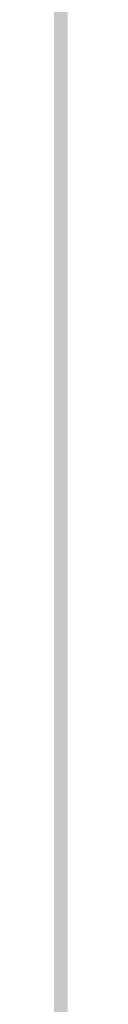
# Model space of a CAD drawing. Units: inches. Extents: x 2083 to 3317, y 1141 to 2115.
# Tile 182 of 256: x 3126.9594 to 3126.95969, y 1263.29018 to 1263.35483. Entities that reach past the tile are written whole.
import ezdxf

# ---------------------------------------------------------------- set-up
doc = ezdxf.new("R2010")
doc.units = ezdxf.units.IN
doc.layers.add('A-ANNO-DIMS', color=2, linetype='Continuous', lineweight=18)
doc.layers.add('A-WALL-PATT', color=251, linetype='Continuous', lineweight=13, true_color=0x636466)
doc.styles.get("Standard").update_dxf_attribs({"font": 'arial.ttf'})
doc.dimstyles.new('ISO-25', dxfattribs={"dimtxt": 12, "dimasz": 12, "dimexe": 1.25, "dimexo": 0.625, "dimtad": 1, "dimlunit": 3, "dimtxsty": 'Standard', "dimcen": 2.5, "dimadec": 0, "dimazin": 0, "dimtfac": 1, "dimtmove": 0, "dimatfit": 3, "dimfxl": 1, "dimarcsym": 0})

# ---------------------------------------------------------------- blocks, each defined once
blk = doc.blocks.new('*D26')
at = {"layer": 'A-ANNO-DIMS', "color": 0, "lineweight": -2, "transparency": 16777216}
for p, q in [((3088.985844, 1274.915092), (3088.985844, 1270.951963)), ((3111.240037, 1274.915092), (3111.240037, 1270.951963)), ((3076.985844, 1272.201963), (2840.262447, 1272.201963)), ((3111.240037, 1272.201963), (3088.985844, 1272.201963)), ((3123.240037, 1272.201963), (3135.240037, 1272.201963))]:
    blk.add_line(p, q, dxfattribs=at)
at = {"layer": 'A-ANNO-DIMS', "color": 0, "transparency": 16777216}
for points in [[(3076.985844, 1274.201963), (3076.985844, 1270.201963), (3088.985844, 1272.201963)], [(3123.240037, 1274.201963), (3123.240037, 1270.201963), (3111.240037, 1272.201963)]]:
    blk.add_solid(points, dxfattribs=at)
at = {"layer": 'Defpoints', "color": 0, "transparency": 16777216}
for p in [(3088.985844, 1275.540092), (3111.240037, 1275.540092), (3088.985844, 1272.201963)]:
    blk.add_point(p, dxfattribs=at)
at = {"layer": 'A-ANNO-DIMS', "color": 0, "transparency": 16777216, "insert": (2952.624146, 1279.031602), "char_height": 12, "attachment_point": 5}
blk.add_mtext('NIGHTSTAND 1\'-10 1/2" TYP.', dxfattribs=at)
blk = doc.blocks.new('*D27')
at = {"layer": 'A-ANNO-DIMS', "color": 0, "lineweight": -2, "transparency": 16777216}
for p, q in [((3114.578165, 1309.794285), (3114.578165, 1321.794285)), ((3111.865037, 1297.794285), (3115.828165, 1297.794285)), ((3114.578165, 1297.794285), (3114.578165, 1275.540092)), ((3111.865037, 1275.540092), (3115.828165, 1275.540092)), ((3114.578165, 1263.540092), (3114.578165, 1140.988591))]:
    blk.add_line(p, q, dxfattribs=at)
at = {"layer": 'A-ANNO-DIMS', "color": 0, "transparency": 16777216}
for points in [[(3112.578165, 1309.794285), (3116.578165, 1309.794285), (3114.578165, 1297.794285)], [(3112.578165, 1263.540092), (3116.578165, 1263.540092), (3114.578165, 1275.540092)]]:
    blk.add_solid(points, dxfattribs=at)
at = {"layer": 'Defpoints', "color": 0, "transparency": 16777216}
for p in [(3111.240037, 1297.794285), (3111.240037, 1275.540092), (3114.578165, 1275.540092)]:
    blk.add_point(p, dxfattribs=at)
at = {"layer": 'A-ANNO-DIMS', "color": 0, "transparency": 16777216, "insert": (3107.748527, 1196.264342), "char_height": 12, "attachment_point": 5, "rotation": 90}
blk.add_mtext('1\'-10 1/2" TYP.', dxfattribs=at)

msp = doc.modelspace()

# ---------------------------------------------------------------- hatches: boundary and pattern name
at = {"layer": 'A-WALL-PATT'}
h = msp.add_hatch(color=256, dxfattribs=at)
h.dxf.hatch_style = 1
h.paths.add_polyline_path([(3126.959783, 2020.76136), (2748.959783, 2020.76136), (2604.959783, 2020.76136), (2226.959783, 2020.76136), (2226.959783, 1702.76136), (2466.959783, 1702.76136), (2466.959783, 1582.76136), (2418.959783, 1582.76136), (2418.959783, 1477.76136), (2226.959783, 1477.76136), (2226.959783, 1263.26136), (2544.959783, 1263.26136), (2544.959783, 1411.76136), (2604.959783, 1411.76136), (2685.959783, 1411.76136), (2685.959783, 1420.76136), (2604.959783, 1420.76136), (2604.959783, 1573.76136), (2604.959783, 1702.76136), (2604.959783, 2011.76136), (2748.959783, 2011.76136), (2748.959783, 1702.76136), (2862.959783, 1702.76136), (2862.959783, 1621.76136), (2871.959783, 1621.76136), (2871.959783, 1702.76136), (2883.959783, 1702.76136), (2883.959783, 1706.939459, -0.026459), (2883.959783, 1711.76136), (2757.959783, 1711.76136), (2757.959783, 1807.76136), (2787.959783, 1807.76136), (2787.959783, 1812.26136), (2757.959783, 1812.26136), (2757.959783, 2011.76136), (2877.959783, 2011.76136), (2877.959783, 1812.26136), (2847.959783, 1812.26136), (2847.959783, 1807.76136), (2889.835742, 1807.76136), (2889.835742, 1812.26136), (2882.459783, 1812.26136), (2882.459783, 2011.76136), (3117.959783, 2011.76136), (3117.959783, 1812.26136), (2937.835742, 1812.26136), (2937.835742, 1807.76136), (2995.709783, 1807.76136), (2995.709783, 1796.117666), (3000.209783, 1796.117666), (3000.209783, 1807.76136), (3117.959783, 1807.76136), (3117.959783, 1711.76136), (3000.209783, 1711.76136), (3000.209783, 1760.117666), (2998.572705, 1760.117666, -0.020711), (2995.709783, 1760.117666), (2995.709783, 1711.76136), (2931.959783, 1711.76136), (2931.959783, 1702.76136), (3126.959783, 1702.76136)])
h.paths.add_polyline_path([(2471.459783, 2011.76136), (2471.459783, 1810.01136), (2462.716936, 1810.01136), (2462.716936, 1805.51136), (2505.959783, 1805.51136), (2505.959783, 1810.01136), (2475.959783, 1810.01136), (2475.959783, 2011.76136), (2595.959783, 2011.76136), (2595.959783, 1810.01136), (2565.959783, 1810.01136), (2565.959783, 1805.51136), (2595.959783, 1805.51136), (2595.959783, 1711.76136), (2235.959783, 1711.76136), (2235.959783, 1805.51136), (2353.709783, 1805.51136), (2353.709783, 1796.054162), (2358.209783, 1796.054162), (2358.209783, 1805.51136), (2414.716936, 1805.51136), (2414.716936, 1810.01136), (2235.959783, 1810.01136), (2235.959783, 2011.76136)], flags=16)
h.paths.add_polyline_path([(2270.204734, 1994.610008), (2270.204734, 1970.610008), (2246.204734, 1970.610008), (2246.204734, 1994.610008)], flags=0)
edge = h.paths.add_edge_path(flags=0)
edge.add_ellipse((2332.027391, 1899.798176), major_axis=(-3.042994, 3.042994), ratio=0.16825245, start_angle=-161.332166, end_angle=-156.307114, ccw=False)
edge.add_ellipse((2333.082037, 1898.74353), major_axis=(-1.054646, 1.054646), ratio=0.4535321, start_angle=-123.371019, end_angle=-94.159107)
edge = h.paths.add_edge_path(flags=0)
edge.add_ellipse((2332.027391, 1968.87629), major_axis=(3.042994, 3.042994), ratio=0.16825245, start_angle=18.667834, end_angle=23.692886)
edge.add_spline(control_points=[(2332.925596, 1970.691105), (2332.226768, 1970.3361), (2330.893709, 1969.658905), (2328.41308, 1970.932138), (2327.203934, 1967.748712), (2324.709596, 1969.955589), (2322.532822, 1967.012354), (2320.012846, 1971.295812), (2317.680308, 1968.157845), (2316.040526, 1967.102047), (2315.426904, 1966.809602)], knot_values=[0, 0, 0, 0, 2.267059, 4.324559, 6.685584, 8.878641, 11.121502, 14.300359, 17.755284, 19.732645, 19.732645, 19.732645, 19.732645], degree=3, periodic=0)
edge.add_ellipse((2332.027391, 1968.87629), major_axis=(3.042994, 3.042994), ratio=0.16825245, start_angle=18.667834, end_angle=23.692886, ccw=False)
edge.add_ellipse((2333.082037, 1969.930936), major_axis=(1.054646, 1.054646), ratio=0.4535321, start_angle=56.628981, end_angle=85.840893, ccw=False)
edge = h.paths.add_edge_path(flags=0)
edge.add_spline(control_points=[(2296.428287, 1967.987908), (2293.627804, 1965.336314), (2287.703624, 1959.727094), (2299.74386, 1949.995699), (2294.532591, 1935.668528), (2290.573228, 1920.603512), (2293.394124, 1909.973691), (2296.185407, 1904.966543)], knot_values=[0.099185, 0.099185, 0.099185, 0.099185, 0.345301, 0.619822, 0.982653, 1.386093, 1.810555, 1.810555, 1.810555, 1.810555], degree=3, periodic=0)
edge.add_spline(control_points=[(2296.185407, 1904.966543), (2297.383582, 1902.6193), (2298.000969, 1901.949312), (2298.55297, 1901.468155)], knot_values=[0.006246, 0.006246, 0.006246, 0.006246, 0.055476, 0.055476, 0.055476, 0.055476], degree=3, periodic=0)
edge.add_spline(control_points=[(2298.55297, 1901.468155), (2297.258612, 1900.923224), (2295.225294, 1900.232126), (2293.060229, 1900.614205), (2292.101423, 1900.788415), (2292.089578, 1900.790568)], knot_values=[0.312835, 0.312835, 0.312835, 0.312835, 0.40178, 0.474987, 0.475903, 0.475903, 0.475903, 0.475903], degree=3, periodic=0)
edge.add_arc((2292.793646, 1904.664109), 3.937008, 215.420897, 259.698179, ccw=False)
edge.add_spline(control_points=[(2289.585314, 1902.382304), (2289.476652, 1902.535087), (2289.36848, 1902.688035), (2289.260865, 1902.84117)], knot_values=[0.102872, 0.102872, 0.102872, 0.102872, 0.116896, 0.116896, 0.116896, 0.116896], degree=3, periodic=0)
edge.add_spline(control_points=[(2289.260865, 1902.84117), (2288.686604, 1902.550192), (2287.640048, 1902.019902), (2285.881337, 1901.873954), (2283.852972, 1901.504352), (2281.719987, 1899.710538), (2278.466991, 1899.492942), (2276.157136, 1901.883202), (2272.258953, 1899.804071), (2267.777605, 1901.843183), (2262.243882, 1900.184033), (2257.414927, 1901.782061), (2254.318374, 1900.72612), (2253.178285, 1900.337343)], knot_values=[0, 0, 0, 0, 1.907977, 3.477176, 5.261074, 7.972851, 11.680248, 13.717921, 16.939592, 22.789562, 27.502503, 33.595215, 37.145618, 37.145618, 37.145618, 37.145618], degree=3, periodic=0)
edge.add_line((2253.178285, 1900.337343), (2250.24424, 1902.84117))
edge.add_line((2250.24424, 1902.84117), (2250.24424, 1965.833296))
edge.add_line((2250.24424, 1965.833296), (2253.178285, 1968.337123))
edge.add_spline(control_points=[(2253.178285, 1968.337123), (2254.318374, 1967.948346), (2257.414927, 1966.892405), (2262.243882, 1968.490433), (2267.777605, 1966.831283), (2271.52673, 1968.537217), (2273.875914, 1967.828289), (2274.206701, 1967.727642)], knot_values=[0, 0, 0, 0, 0.09018, 0.244935, 0.364644, 0.513233, 0.537855, 0.537855, 0.537855, 0.537855], degree=3, periodic=0)
edge.add_arc((2274.352887, 1963.793349), 3.937008, 72.051134, 92.127949, ccw=False)
edge.add_arc((2281.296933, 1985.230003), 18.596298, 252.0511336, 288.5657217)
edge.add_arc((2292.316717, 1956.02888), 12.646081, 71.0267879, 113.7782184, ccw=False)
edge = h.paths.add_edge_path(flags=0)
edge.add_spline(control_points=[(2274.899415, 1951.856195), (2275.066156, 1951.616592), (2275.232687, 1951.376588), (2275.397987, 1951.135855)], knot_values=[1.409916, 1.409916, 1.409916, 1.409916, 1.43159, 1.43159, 1.43159, 1.43159], degree=3, periodic=0)
edge.add_spline(control_points=[(2275.397987, 1951.135855), (2275.792106, 1950.561885), (2276.179231, 1949.983774), (2276.545546, 1949.397103)], knot_values=[1.358238, 1.358238, 1.358238, 1.358238, 1.409916, 1.409916, 1.409916, 1.409916], degree=3, periodic=0)
edge.add_line((2276.545546, 1949.397103), (2277.437289, 1947.862185))
edge.add_spline(control_points=[(2277.437289, 1947.862185), (2276.303834, 1945.673115), (2274.639698, 1942.426882), (2274.631615, 1938.0939), (2272.799124, 1930.85155), (2274.356426, 1943.897046), (2275.947681, 1947.923356), (2276.545546, 1949.397103)], knot_values=[0.005632, 0.005632, 0.005632, 0.005632, 0.186014, 0.266002, 0.357087, 0.59639, 0.739732, 0.739732, 0.739732, 0.739732], degree=3, periodic=0)
edge.add_spline(control_points=[(2276.545546, 1949.397103), (2276.179231, 1949.983774), (2275.792106, 1950.561885), (2275.397987, 1951.135855)], knot_values=[1.358238, 1.358238, 1.358238, 1.358238, 1.409916, 1.409916, 1.409916, 1.409916], degree=3, periodic=0)
edge.add_spline(control_points=[(2275.397987, 1951.135855), (2274.9425, 1950.080452), (2274.20776, 1948.025272), (2273.934602, 1944.851477), (2272.468534, 1937.627489), (2273.466216, 1945.696466), (2274.700615, 1951.059472), (2274.899415, 1951.856195)], knot_values=[0.104364, 0.104364, 0.104364, 0.104364, 0.189636, 0.269624, 0.36071, 0.600013, 0.644622, 0.644622, 0.644622, 0.644622], degree=3, periodic=0)
h.paths.add_polyline_path([(2269.167514, 1963.127573, -0.357527), (2268.170633, 1960.97637, -0.092561), (2268.170633, 1939.436325, -0.357527), (2269.167514, 1937.285122, -0.357527), (2267.01631, 1938.282002, -0.164785), (2254.685581, 1938.282002, -0.357527), (2252.534378, 1937.285122, -0.357527), (2253.531259, 1939.436325, -0.092561), (2253.531259, 1960.97637, -0.357527), (2252.534378, 1963.127573, -0.357527), (2254.685581, 1962.130692, -0.164785), (2267.01631, 1962.130692, -0.357527)], flags=0)
h.paths.add_polyline_path([(2248.874068, 1967.8018), (2248.874068, 1957.02771), (2249.457783, 1957.02771), (2249.457783, 1911.646756), (2248.874068, 1911.646756), (2248.874068, 1900.872666), (2246.511863, 1900.872666, 0.197327), (2244.149658, 1902.456873), (2244.149658, 1966.217592, 0.197327), (2246.511863, 1967.8018)], flags=0)
h.paths.add_polyline_path([(2269.167514, 1931.389344, -0.357527), (2268.170633, 1929.238141, -0.092561), (2268.170633, 1907.698096, -0.357527), (2269.167514, 1905.546893, -0.357527), (2267.01631, 1906.543774, -0.164785), (2254.685581, 1906.543774, -0.357527), (2252.534378, 1905.546893, -0.357527), (2253.531259, 1907.698096, -0.092561), (2253.531259, 1929.238141, -0.357527), (2252.534378, 1931.389344, -0.357527), (2254.685581, 1930.392463, -0.164785), (2267.01631, 1930.392463, -0.357527)], flags=0)
edge = h.paths.add_edge_path(flags=0)
edge.add_spline(control_points=[(2276.196858, 1906.723702), (2276.168144, 1909.028928), (2276.114049, 1913.371852), (2270.598417, 1924.924978), (2273.905175, 1919.012779), (2275.921711, 1916.262063), (2275.47457, 1912.402149), (2277.257874, 1910.380621), (2276.696044, 1908.225036), (2276.646218, 1906.813023), (2276.617825, 1906.008407)], knot_values=[0, 0, 0, 0, 8.61026, 16.221274, 18.843057, 23.804898, 27.440828, 29.356102, 31.203478, 33.650687, 33.650687, 33.650687, 33.650687], degree=3, periodic=0)
edge.add_spline(control_points=[(2276.617825, 1906.008407), (2276.623313, 1905.624144), (2276.497738, 1904.628661), (2275.441779, 1903.854725), (2274.937314, 1903.08045), (2274.85908, 1902.84117)], knot_values=[0.156488, 0.156488, 0.156488, 0.156488, 0.184398, 0.231376, 0.250598, 0.250598, 0.250598, 0.250598], degree=3, periodic=0)
edge.add_line((2274.85908, 1902.84117), (2276.50598, 1902.84117))
edge.add_spline(control_points=[(2276.50598, 1902.84117), (2276.788308, 1903.08494), (2277.665071, 1904.125196), (2278.249538, 1904.340738), (2277.653872, 1908.527387), (2278.15567, 1906.227808), (2278.100464, 1905.285948), (2278.846675, 1904.069005), (2277.856785, 1903.414948), (2277.874191, 1902.99105), (2277.903562, 1902.84117)], knot_values=[0.059574, 0.059574, 0.059574, 0.059574, 0.080753, 0.103741, 0.16972, 0.176036, 0.207137, 0.240474, 0.262341, 0.27366, 0.27366, 0.27366, 0.27366], degree=3, periodic=0)
edge.add_line((2277.903562, 1902.84117), (2280.029825, 1902.84117))
edge.add_spline(control_points=[(2280.029825, 1902.84117), (2279.888221, 1903.088398), (2279.499257, 1903.981551), (2280.152284, 1905.939349), (2278.103615, 1909.657757), (2279.762395, 1907.185285), (2280.3279, 1904.874861), (2280.485109, 1903.48959), (2281.463269, 1903.249432), (2281.758343, 1902.936497), (2281.834036, 1902.84117)], knot_values=[0.013856, 0.013856, 0.013856, 0.013856, 0.034874, 0.088867, 0.107879, 0.126738, 0.158714, 0.193757, 0.217487, 0.226722, 0.226722, 0.226722, 0.226722], degree=3, periodic=0)
edge.add_spline(control_points=[(2281.834036, 1902.84117), (2281.787535, 1902.826703), (2281.647022, 1902.782988), (2281.395527, 1902.85949), (2281.088077, 1902.985242), (2280.720683, 1903.060902), (2280.333451, 1903.025726), (2280.124767, 1902.898879), (2280.029825, 1902.84117)], knot_values=[0, 0, 0, 0, 0.14413, 0.435517, 0.749276, 1.153046, 1.548371, 1.878348, 1.878348, 1.878348, 1.878348], degree=3, periodic=0)
edge.add_line((2280.029825, 1902.84117), (2277.903562, 1902.84117))
edge.add_spline(control_points=[(2277.903562, 1902.84117), (2277.892855, 1902.795855), (2277.865396, 1902.679637), (2277.607479, 1902.687483), (2277.27405, 1902.8007), (2276.837921, 1902.619775), (2276.583807, 1902.789261), (2276.50598, 1902.84117)], knot_values=[0, 0, 0, 0, 0.127189, 0.326199, 0.628009, 1.24357, 1.515331, 1.515331, 1.515331, 1.515331], degree=3, periodic=0)
edge.add_line((2276.50598, 1902.84117), (2274.85908, 1902.84117))
edge.add_spline(control_points=[(2274.85908, 1902.84117), (2274.814437, 1902.898587), (2274.72513, 1903.013446), (2274.493477, 1903.118968), (2274.244285, 1902.960539), (2273.937121, 1903.184942), (2273.614039, 1902.983143), (2273.408316, 1902.883045), (2273.322254, 1902.84117)], knot_values=[0, 0, 0, 0, 0.21843, 0.436957, 0.687977, 0.990379, 1.398396, 1.69185, 1.69185, 1.69185, 1.69185], degree=3, periodic=0)
edge.add_spline(control_points=[(2273.322254, 1902.84117), (2273.61674, 1903.445692), (2274.273998, 1904.538253), (2276.027239, 1904.573702), (2276.206963, 1906.583637), (2276.196858, 1906.723702)], knot_values=[0.012227, 0.012227, 0.012227, 0.012227, 0.059472, 0.106218, 0.134458, 0.134458, 0.134458, 0.134458], degree=3, periodic=0)
h.paths.add_polyline_path([(2270.776054, 1897.789828), (2270.776054, 1873.789828), (2246.776054, 1873.789828), (2246.776054, 1897.789828)], flags=0)
h.paths.add_polyline_path([(2353.709783, 1760.005059), (2353.709783, 1760.054162), (2358.209783, 1760.054162, -0.033729)], flags=0)
h.paths.add_polyline_path([(2321.819119, 1737.529186), (2341.995327, 1737.529186, -0.414214), (2343.203273, 1736.321241), (2343.203273, 1721.020596, -0.414214), (2341.995327, 1719.812651), (2321.819119, 1719.812651, -0.414214), (2320.611173, 1721.020596), (2320.611173, 1736.321241, -0.414214)], flags=0)
h.paths.add_polyline_path([(2324.23501, 1736.321241), (2339.579436, 1736.321241, -0.414214), (2341.995327, 1733.905349), (2341.995327, 1725.44973, -0.414214), (2339.579436, 1723.033839), (2333.680588, 1723.033839), (2333.845317, 1722.045467, -0.870646), (2335.425399, 1721.825893, -0.767327), (2333.922694, 1721.423245), (2331.291024, 1721.423245, -0.767327), (2329.788319, 1721.825893, -0.870646), (2331.368401, 1722.045467), (2331.53313, 1723.033839), (2324.23501, 1723.033839, -0.414214), (2321.819119, 1725.44973), (2321.819119, 1733.905349, -0.414214)], flags=0)
h.paths.add_polyline_path([(2570.483789, 1928.615444), (2589.683789, 1928.615444), (2590.168829, 1928.615444), (2590.168829, 1904.993397), (2570.483789, 1904.993397)], flags=0)
h.paths.add_polyline_path([(2574.447324, 1927.263822, -1), (2572.828836, 1927.263822, -1)], flags=0)
h.paths.add_polyline_path([(2573.089867, 1926.940877), (2573.925032, 1927.776042), (2574.147743, 1927.553332), (2573.312577, 1926.718166)], flags=0)
h.paths.add_polyline_path([(2578.779065, 1919.729618, -1), (2571.591663, 1919.729618, -1)], flags=0)
h.paths.add_polyline_path([(2578.385364, 1919.729618, -1), (2571.985364, 1919.729618, -1)], flags=0)
h.paths.add_polyline_path([(2331.595764, 1729.476216, -1), (2333.617954, 1729.476216, -1)], flags=0)
h.paths.add_polyline_path([(2578.034228, 1927.263822, -1), (2576.41574, 1927.263822, -1)], flags=0)
h.paths.add_polyline_path([(2576.688851, 1927.531089), (2576.911562, 1927.753799), (2577.746728, 1926.918634), (2577.524017, 1926.695923)], flags=0)
h.paths.add_polyline_path([(2578.139065, 1909.859539, -1), (2572.231663, 1909.859539, -1)], flags=0)
h.paths.add_polyline_path([(2577.745364, 1909.859539, -1), (2572.625364, 1909.859539, -1)], flags=0)
h.paths.add_polyline_path([(2583.797718, 1927.263822, -1), (2582.179229, 1927.263822, -1)], flags=0)
h.paths.add_polyline_path([(2582.718649, 1927.753799), (2583.553814, 1926.918634), (2583.331103, 1926.695923), (2582.495938, 1927.531089)], flags=0)
h.paths.add_polyline_path([(2582.495938, 1927.531089), (2582.718649, 1927.753799), (2583.553814, 1926.918634), (2583.331103, 1926.695923)], flags=0)
h.paths.add_polyline_path([(2587.739065, 1920.529618, -1), (2581.831663, 1920.529618, -1)], flags=0)
h.paths.add_polyline_path([(2587.345364, 1920.529618, -1), (2582.225364, 1920.529618, -1)], flags=0)
h.paths.add_polyline_path([(2587.384622, 1927.263822, -1), (2585.766133, 1927.263822, -1)], flags=0)
h.paths.add_polyline_path([(2586.081993, 1926.980247), (2586.917158, 1927.815412), (2587.139869, 1927.592702), (2586.304703, 1926.757536)], flags=0)
h.paths.add_polyline_path([(2588.379065, 1910.659539, -1), (2581.191663, 1910.659539, -1)], flags=0)
h.paths.add_polyline_path([(2587.985364, 1910.659539, -1), (2581.585364, 1910.659539, -1)], flags=0)
h.paths.add_polyline_path([(2417.167729, 1729.477895), (2437.343937, 1729.477895, -0.414214), (2438.551883, 1728.26995), (2438.551883, 1712.969306, -0.414214), (2437.343937, 1711.76136), (2417.167729, 1711.76136, -0.414214), (2415.959783, 1712.969306), (2415.959783, 1728.26995, -0.414214)], flags=0)
h.paths.add_polyline_path([(2419.58362, 1728.26995), (2434.928046, 1728.26995, -0.414214), (2437.343937, 1725.854059), (2437.343937, 1717.39844, -0.414214), (2434.928046, 1714.982548), (2429.029199, 1714.982548), (2429.193927, 1713.994176, -0.870646), (2430.774009, 1713.774603, -0.767327), (2429.271304, 1713.371954), (2426.639634, 1713.371954, -0.767327), (2425.136929, 1713.774603, -0.870646), (2426.717011, 1713.994176), (2426.88174, 1714.982548), (2419.58362, 1714.982548, -0.414214), (2417.167729, 1717.39844), (2417.167729, 1725.854059, -0.414214)], flags=0)
h.paths.add_polyline_path([(2419.58362, 1728.26995), (2434.928046, 1728.26995, -0.414214), (2437.343937, 1725.854059), (2437.343937, 1717.39844, -0.414214), (2434.928046, 1714.982548), (2429.029199, 1714.982548), (2428.358118, 1719.009034), (2427.552821, 1719.009034), (2426.88174, 1714.982548), (2419.58362, 1714.982548, -0.414214), (2417.167729, 1717.39844), (2417.167729, 1725.854059, -0.414214)], flags=0)
h.paths.add_polyline_path([(2426.944374, 1721.424925, -1), (2428.966564, 1721.424925, -1)], flags=0)
h.paths.add_polyline_path([(2475.959783, 1702.76136), (2595.959783, 1702.76136), (2595.959783, 1582.76136), (2475.959783, 1582.76136)], flags=16)
h.paths.add_polyline_path([(2427.959783, 1573.76136), (2595.959783, 1573.76136), (2595.959783, 1468.76136), (2595.959783, 1420.76136), (2384.459783, 1420.76136), (2384.459783, 1468.76136), (2427.959783, 1468.76136)], flags=16)
h.paths.add_polyline_path([(2379.959783, 1468.76136), (2379.959783, 1420.76136), (2235.959783, 1420.76136), (2235.959783, 1468.76136)], flags=16)
h.paths.add_polyline_path([(2317.815996, 1466.695767), (2337.992205, 1466.695767, -0.414214), (2339.20015, 1465.487821), (2339.20015, 1450.187177, -0.414214), (2337.992205, 1448.979232), (2317.815996, 1448.979232, -0.414214), (2316.608051, 1450.187177), (2316.608051, 1465.487821, -0.414214)], flags=0)
h.paths.add_polyline_path([(2320.231887, 1465.487821), (2335.576313, 1465.487821, -0.414214), (2337.992205, 1463.07193), (2337.992205, 1454.616311, -0.414214), (2335.576313, 1452.20042), (2329.677466, 1452.20042), (2329.842195, 1451.212047, -0.870646), (2331.422276, 1450.992474, -0.767327), (2329.919571, 1450.589826), (2327.287902, 1450.589826, -0.767327), (2325.785197, 1450.992474, -0.870646), (2327.365278, 1451.212047), (2327.530007, 1452.20042), (2320.231887, 1452.20042, -0.414214), (2317.815996, 1454.616311), (2317.815996, 1463.07193, -0.414214)], flags=0)
h.paths.add_polyline_path([(2320.231887, 1465.487821), (2335.576313, 1465.487821, -0.414214), (2337.992205, 1463.07193), (2337.992205, 1454.616311, -0.414214), (2335.576313, 1452.20042), (2329.677466, 1452.20042), (2329.006385, 1456.226905), (2328.201088, 1456.226905), (2327.530007, 1452.20042), (2320.231887, 1452.20042, -0.414214), (2317.815996, 1454.616311), (2317.815996, 1463.07193, -0.414214)], flags=0)
h.paths.add_polyline_path([(2327.592641, 1458.642796, -1), (2329.614832, 1458.642796, -1)], flags=0)
h.paths.add_polyline_path([(2244.411744, 1433.340453), (2241.920945, 1433.340453, -0.414214), (2240.017856, 1435.243542), (2240.017856, 1440.952808, -0.414211), (2241.920925, 1442.855897), (2244.411744, 1442.855897, -1.976472)], flags=0)
h.paths.add_polyline_path([(2245.356888, 1434.397536, -0.414214), (2245.356888, 1441.798814, -2.144098)], flags=0)
h.paths.add_polyline_path([(2535.959783, 1416.26136), (2535.959783, 1272.26136), (2235.959783, 1272.26136), (2235.959783, 1416.26136)], flags=16)
h.paths.add_polyline_path([(2260.119561, 1384.292841), (2260.119561, 1362.038649), (2237.865369, 1362.038649), (2237.865369, 1384.292841)], flags=0)
edge = h.paths.add_edge_path(flags=0)
edge.add_line((2318.251847, 1362.093298), (2318.145797, 1362.000973))
edge.add_ellipse((2317.445116, 1360.431044), major_axis=(2.82164, 2.82164), ratio=0.16825245, start_angle=18.667834, end_angle=20.948127, ccw=False)
edge.add_ellipse((2318.423045, 1361.408974), major_axis=(0.977929, 0.977929), ratio=0.4535321, start_angle=56.628981, end_angle=70.226201, ccw=False)
edge = h.paths.add_edge_path(flags=0)
edge.add_line((2319.10737, 1295.571078), (2319.015044, 1295.677128))
edge.add_ellipse((2317.445116, 1296.377809), major_axis=(-2.82164, 2.82164), ratio=0.16825245, start_angle=-161.332166, end_angle=-159.051873, ccw=False)
edge.add_ellipse((2318.423045, 1295.39988), major_axis=(-0.977929, 0.977929), ratio=0.4535321, start_angle=-123.371019, end_angle=-109.773799)
edge = h.paths.add_edge_path(flags=0)
edge.add_spline(control_points=[(2284.210349, 1301.170219), (2284.580688, 1300.444719), (2284.891189, 1299.892024), (2285.159553, 1299.461018)], knot_values=[0.039066, 0.039066, 0.039066, 0.039066, 0.055476, 0.055476, 0.055476, 0.055476], degree=3, periodic=0)
edge.add_line((2285.159553, 1299.461018), (2284.210349, 1301.170219))
edge = h.paths.add_edge_path(flags=0)
edge.add_line((2280.412458, 1297.298013), (2283.369991, 1297.036122))
edge.add_line((2283.369991, 1297.036122), (2286.40569, 1297.92631))
edge.add_spline(control_points=[(2286.40569, 1297.92631), (2285.305487, 1297.463119), (2284.344777, 1297.129151), (2283.369991, 1297.036122)], knot_values=[0.394369, 0.394369, 0.394369, 0.394369, 0.475903, 0.475903, 0.475903, 0.475903], degree=3, periodic=0)
edge.add_spline(control_points=[(2283.369991, 1297.036122), (2283.28139, 1297.027666), (2282.316289, 1296.957336), (2281.312502, 1297.134479), (2280.423441, 1297.296016), (2280.412458, 1297.298013)], knot_values=[0.312835, 0.312835, 0.312835, 0.312835, 0.320246, 0.393453, 0.394369, 0.394369, 0.394369, 0.394369], degree=3, periodic=0)
edge = h.paths.add_edge_path(flags=0)
edge.add_line((2284.435561, 1359.607285), (2280.446291, 1355.328047))
edge.add_line((2280.446291, 1355.328047), (2279.579987, 1351.017754))
edge.add_line((2279.579987, 1351.017754), (2282.412974, 1346.580433))
edge.add_spline(control_points=[(2282.412974, 1346.580433), (2283.153331, 1345.589236), (2284.252896, 1344.028897), (2284.801037, 1342.387167), (2284.935162, 1341.805544)], knot_values=[1.240098, 1.240098, 1.240098, 1.240098, 1.332892, 1.382712, 1.382712, 1.382712, 1.382712], degree=3, periodic=0)
edge.add_spline(control_points=[(2284.935162, 1341.805544), (2285.319108, 1340.1406), (2285.233029, 1338.409204), (2284.909938, 1336.654122)], knot_values=[1.097484, 1.097484, 1.097484, 1.097484, 1.240098, 1.240098, 1.240098, 1.240098], degree=3, periodic=0)
edge.add_spline(control_points=[(2284.909938, 1336.654122), (2284.586848, 1334.89904), (2284.026745, 1333.120272), (2283.462644, 1331.360585)], knot_values=[0.95487, 0.95487, 0.95487, 0.95487, 1.097484, 1.097484, 1.097484, 1.097484], degree=3, periodic=0)
edge.add_line((2283.462644, 1331.360585), (2281.890376, 1326.153357))
edge.add_line((2281.890376, 1326.153357), (2280.756259, 1321.056089))
edge.add_line((2280.756259, 1321.056089), (2280.299205, 1316.001977))
edge.add_line((2280.299205, 1316.001977), (2280.715933, 1310.950068))
edge.add_line((2280.715933, 1310.950068), (2282.028094, 1305.972137))
edge.add_line((2282.028094, 1305.972137), (2284.210349, 1301.170219))
edge.add_spline(control_points=[(2284.210349, 1301.170219), (2283.340731, 1302.730185), (2282.611904, 1304.336493), (2282.028094, 1305.972137)], knot_values=[0.099185, 0.099185, 0.099185, 0.099185, 0.241799, 0.241799, 0.241799, 0.241799], degree=3, periodic=0)
edge.add_spline(control_points=[(2282.028094, 1305.972137), (2281.444283, 1307.60778), (2281.005489, 1309.272759), (2280.715933, 1310.950068)], knot_values=[0.241799, 0.241799, 0.241799, 0.241799, 0.384413, 0.384413, 0.384413, 0.384413], degree=3, periodic=0)
edge.add_spline(control_points=[(2280.715933, 1310.950068), (2280.433241, 1312.587613), (2280.289386, 1314.276959), (2280.298894, 1315.962032), (2280.299205, 1316.001977)], knot_values=[0.384413, 0.384413, 0.384413, 0.384413, 0.523647, 0.527028, 0.527028, 0.527028, 0.527028], degree=3, periodic=0)
edge.add_spline(control_points=[(2280.299205, 1316.001977), (2280.312326, 1317.686955), (2280.477871, 1319.367926), (2280.756259, 1321.056089)], knot_values=[0.527028, 0.527028, 0.527028, 0.527028, 0.669642, 0.669642, 0.669642, 0.669642], degree=3, periodic=0)
edge.add_spline(control_points=[(2280.756259, 1321.056089), (2281.034648, 1322.744252), (2281.42588, 1324.439608), (2281.890376, 1326.153357)], knot_values=[0.669642, 0.669642, 0.669642, 0.669642, 0.812256, 0.812256, 0.812256, 0.812256], degree=3, periodic=0)
edge.add_spline(control_points=[(2281.890376, 1326.153357), (2282.264383, 1327.533251), (2282.78787, 1329.26181), (2283.352751, 1331.01778), (2283.462644, 1331.360585)], knot_values=[0.812256, 0.812256, 0.812256, 0.812256, 0.927087, 0.95487, 0.95487, 0.95487, 0.95487], degree=3, periodic=0)
edge.add_line((2283.462644, 1331.360585), (2284.909938, 1336.654122))
edge.add_line((2284.909938, 1336.654122), (2284.935162, 1341.805544))
edge.add_line((2284.935162, 1341.805544), (2282.412974, 1346.580433))
edge.add_spline(control_points=[(2282.412974, 1346.580433), (2281.275127, 1348.103792), (2280.078447, 1349.570318), (2279.579987, 1351.017754)], knot_values=[1.382712, 1.382712, 1.382712, 1.382712, 1.525326, 1.525326, 1.525326, 1.525326], degree=3, periodic=0)
edge.add_spline(control_points=[(2279.579987, 1351.017754), (2279.443282, 1351.414721), (2279.136312, 1352.856922), (2279.73519, 1354.290385), (2280.446291, 1355.328047)], knot_values=[1.525326, 1.525326, 1.525326, 1.525326, 1.564439, 1.667941, 1.667941, 1.667941, 1.667941], degree=3, periodic=0)
edge.add_spline(control_points=[(2280.446291, 1355.328047), (2281.426113, 1356.757835), (2282.930837, 1358.18256), (2284.435561, 1359.607285)], knot_values=[1.667941, 1.667941, 1.667941, 1.667941, 1.810555, 1.810555, 1.810555, 1.810555], degree=3, periodic=0)
edge.add_arc((2280.623075, 1348.518181), 11.72618, 71.0267879, 113.7782184)
edge.add_arc((2270.404892, 1375.595156), 17.243567, 252.0511336, 288.5657217, ccw=False)
edge.add_arc((2263.965969, 1355.717847), 3.650622, 72.051134, 92.127949)
edge.add_arc((2263.965969, 1355.717847), 3.650622, 92.127949, 177.98513)
edge.add_spline(control_points=[(2260.317604, 1355.846199), (2260.260417, 1354.220668), (2260.551278, 1350.186547), (2262.999344, 1346.766251), (2264.472741, 1344.649024)], knot_values=[1.43159, 1.43159, 1.43159, 1.43159, 1.564144, 1.770695, 1.770695, 1.770695, 1.770695], degree=3, periodic=0)
edge.add_line((2264.472741, 1344.649024), (2264.93559, 1343.98253))
edge.add_spline(control_points=[(2263.801044, 1340.248105), (2263.843238, 1340.514088), (2264.067244, 1341.756465), (2264.512693, 1343.002453), (2264.935047, 1343.981083)], knot_values=[0.53657, 0.53657, 0.53657, 0.53657, 0.559349, 0.644622, 0.644622, 0.644622, 0.644622], degree=3, periodic=0)
edge.add_spline(control_points=[(2264.935047, 1343.981083), (2265.117771, 1343.714975), (2265.298875, 1343.447906), (2265.476756, 1343.179365)], knot_values=[1.384077, 1.384077, 1.384077, 1.384077, 1.409916, 1.409916, 1.409916, 1.409916], degree=3, periodic=0)
edge.add_spline(control_points=[(2265.476756, 1343.179365), (2265.654637, 1342.910823), (2265.829296, 1342.64081), (2265.99913, 1342.368812)], knot_values=[1.358238, 1.358238, 1.358238, 1.358238, 1.384077, 1.384077, 1.384077, 1.384077], degree=3, periodic=0)
edge.add_line((2265.99913, 1342.368812), (2266.826006, 1340.945547))
edge.add_spline(control_points=[(2266.826006, 1340.945547), (2268.894401, 1337.089691), (2271.398173, 1325.843001), (2270.516164, 1310.568557), (2275.919376, 1301.860609), (2277.789511, 1299.19945)], knot_values=[0.116896, 0.116896, 0.116896, 0.116896, 0.472987, 1.050969, 1.313793, 1.313793, 1.313793, 1.313793], degree=3, periodic=0)
edge.add_spline(control_points=[(2277.789511, 1299.19945), (2277.839405, 1299.128452), (2277.889428, 1299.057498), (2277.939572, 1298.986584)], knot_values=[0.109884, 0.109884, 0.109884, 0.109884, 0.116896, 0.116896, 0.116896, 0.116896], degree=3, periodic=0)
edge.add_line((2277.939572, 1298.986584), (2277.788849, 1299.199114))
edge.add_spline(control_points=[(2277.788849, 1299.199114), (2277.256582, 1298.929414), (2276.28635, 1298.437902), (2275.039352, 1298.334419), (2274.38333, 1298.238895), (2274.215254, 1298.209338)], knot_values=[33.12187, 33.12187, 33.12187, 33.12187, 35.029056, 36.598255, 37.144827, 37.144827, 37.144827, 37.144827], degree=3, periodic=0)
edge.add_line((2274.215254, 1298.209338), (2273.073147, 1297.892961))
edge.add_spline(control_points=[(2273.073147, 1297.892961), (2272.322936, 1297.579784), (2271.039151, 1296.510508), (2269.248395, 1296.226062), (2268.4231, 1296.374654)], knot_values=[26.532584, 26.532584, 26.532584, 26.532584, 29.198919, 31.839101, 31.839101, 31.839101, 31.839101], degree=3, periodic=0)
edge.add_line((2268.4231, 1296.374654), (2263.878501, 1297.457534))
edge.add_spline(control_points=[(2263.878501, 1297.457534), (2263.556077, 1297.359435), (2261.860306, 1296.838694), (2260.23878, 1297.282407), (2258.933454, 1297.516461)], knot_values=[15.919551, 15.919551, 15.919551, 15.919551, 16.939592, 21.226067, 21.226067, 21.226067, 21.226067], degree=3, periodic=0)
edge.add_line((2258.933454, 1297.516461), (2254.055233, 1297.32901))
edge.add_spline(control_points=[(2254.055233, 1297.32901), (2253.755525, 1297.295815), (2252.113683, 1297.165174), (2250.461869, 1297.544221), (2249.129686, 1297.667882)], knot_values=[5.306517, 5.306517, 5.306517, 5.306517, 6.276435, 10.613034, 10.613034, 10.613034, 10.613034], degree=3, periodic=0)
edge.add_line((2249.129686, 1297.667882), (2244.33165, 1296.877756))
edge.add_line((2244.33165, 1296.877756), (2241.611033, 1299.19945))
edge.add_line((2241.611033, 1299.19945), (2241.611033, 1357.609404))
edge.add_line((2241.611033, 1357.609404), (2244.33165, 1359.931097))
edge.add_line((2244.33165, 1359.931097), (2252.728823, 1359.542692))
edge.add_spline(control_points=[(2252.728823, 1359.542692), (2252.870939, 1359.54644), (2253.30574, 1359.548172), (2253.739845, 1359.514274), (2254.031742, 1359.482426)], knot_values=[0.233291, 0.233291, 0.233291, 0.233291, 0.244935, 0.268927, 0.268927, 0.268927, 0.268927], degree=3, periodic=0)
edge.add_line((2254.031742, 1359.482426), (2259.58719, 1359.41639))
edge.add_spline(control_points=[(2259.58719, 1359.41639), (2260.677068, 1359.628503), (2262.073197, 1359.897003), (2263.523692, 1359.459278), (2263.830417, 1359.365952)], knot_values=[0.422516, 0.422516, 0.422516, 0.422516, 0.513233, 0.537855, 0.537855, 0.537855, 0.537855], degree=3, periodic=0)
edge.add_arc((2263.965969, 1355.717847), 3.650622, 72.051134, 92.127949, ccw=False)
edge.add_arc((2270.404892, 1375.595156), 17.243567, 252.0511336, 288.5657217)
edge.add_arc((2280.623075, 1348.518181), 11.72618, 71.0267879, 113.7782184, ccw=False)
h.paths.add_polyline_path([(2240.34053, 1359.434715), (2240.34053, 1349.444353), (2240.881785, 1349.444353), (2240.881785, 1307.3645), (2240.34053, 1307.3645), (2240.34053, 1297.374138), (2238.150157, 1297.374138, 0.197327), (2235.959783, 1298.843108), (2235.959783, 1357.965746, 0.197327), (2238.150157, 1359.434715)], flags=0)
h.paths.add_polyline_path([(2259.15779, 1355.1005, -0.357527), (2258.233425, 1353.10578, -0.092561), (2258.233425, 1333.132601, -0.357527), (2259.15779, 1331.13788, -0.357527), (2257.16307, 1332.062246, -0.164785), (2245.729302, 1332.062246, -0.357527), (2243.734582, 1331.13788, -0.357527), (2244.658947, 1333.132601, -0.092561), (2244.658947, 1353.10578, -0.357527), (2243.734582, 1355.1005, -0.357527), (2245.729302, 1354.176135, -0.164785), (2257.16307, 1354.176135, -0.357527)], flags=0)
edge = h.paths.add_edge_path(flags=0)
edge.add_line((2265.99913, 1342.368812), (2266.826006, 1340.945547))
edge.add_line((2266.826006, 1340.945547), (2265.307557, 1337.814066))
edge.add_line((2265.307557, 1337.814066), (2264.358232, 1334.652939))
edge.add_line((2264.358232, 1334.652939), (2264.262012, 1333.799705))
edge.add_spline(control_points=[(2264.262012, 1333.799705), (2264.208357, 1333.187055), (2264.16206, 1332.365525), (2264.007144, 1331.413933), (2263.969049, 1331.201834)], knot_values=[0.464444, 0.464444, 0.464444, 0.464444, 0.516691, 0.531608, 0.531608, 0.531608, 0.531608], degree=3, periodic=0)
edge.add_spline(control_points=[(2263.969049, 1331.201834), (2263.774535, 1330.118873), (2263.42437, 1328.790839), (2263.25742, 1328.530652), (2263.234028, 1328.514612)], knot_values=[0.372682, 0.372682, 0.372682, 0.372682, 0.44885, 0.464444, 0.464444, 0.464444, 0.464444], degree=3, periodic=0)
edge.add_spline(control_points=[(2263.234028, 1328.514612), (2263.096382, 1328.420227), (2263.13117, 1329.301477), (2263.274953, 1330.615749)], knot_values=[0.280919, 0.280919, 0.280919, 0.280919, 0.372682, 0.372682, 0.372682, 0.372682], degree=3, periodic=0)
edge.add_spline(control_points=[(2263.274953, 1330.615749), (2263.418736, 1331.930022), (2263.671515, 1333.677318), (2263.969852, 1335.315027)], knot_values=[0.189157, 0.189157, 0.189157, 0.189157, 0.280919, 0.280919, 0.280919, 0.280919], degree=3, periodic=0)
edge.add_spline(control_points=[(2263.969852, 1335.315027), (2264.100496, 1336.032192), (2264.418783, 1337.621911), (2264.754848, 1338.86443), (2264.947419, 1339.491124)], knot_values=[0.097394, 0.097394, 0.097394, 0.097394, 0.137578, 0.189157, 0.189157, 0.189157, 0.189157], degree=3, periodic=0)
edge.add_spline(control_points=[(2264.947419, 1339.491124), (2265.290017, 1340.606055), (2265.644238, 1341.493996), (2265.99913, 1342.368812)], knot_values=[0.005632, 0.005632, 0.005632, 0.005632, 0.097394, 0.097394, 0.097394, 0.097394], degree=3, periodic=0)
h.paths.add_polyline_path([(2259.15779, 1325.670973, -0.357527), (2258.233425, 1323.676253, -0.092561), (2258.233425, 1303.703073, -0.357527), (2259.15779, 1301.708353, -0.357527), (2257.16307, 1302.632719, -0.164785), (2245.729302, 1302.632719, -0.357527), (2243.734582, 1301.708353, -0.357527), (2244.658947, 1303.703073, -0.092561), (2244.658947, 1323.676253, -0.357527), (2243.734582, 1325.670973, -0.357527), (2245.729302, 1324.746608, -0.164785), (2257.16307, 1324.746608, -0.357527)], flags=0)
edge = h.paths.add_edge_path(flags=0)
edge.add_spline(control_points=[(2261.708938, 1317.311421), (2261.679482, 1317.41758), (2261.761858, 1317.388535), (2262.490736, 1316.089873), (2262.962185, 1315.300897)], knot_values=[14.955861, 14.955861, 14.955861, 14.955861, 16.221274, 18.694826, 18.694826, 18.694826, 18.694826], degree=3, periodic=0)
edge.add_spline(control_points=[(2262.962185, 1315.300897), (2262.990437, 1315.253617), (2263.702096, 1314.067376), (2264.348983, 1313.127153), (2264.730054, 1312.164154)], knot_values=[18.694826, 18.694826, 18.694826, 18.694826, 18.843057, 22.433791, 22.433791, 22.433791, 22.433791], degree=3, periodic=0)
edge.add_spline(control_points=[(2264.730054, 1312.164154), (2264.875565, 1311.796437), (2265.176873, 1310.769807), (2265.143069, 1309.559262), (2265.247736, 1308.824193)], knot_values=[22.433791, 22.433791, 22.433791, 22.433791, 23.804898, 26.172756, 26.172756, 26.172756, 26.172756], degree=3, periodic=0)
edge.add_line((2265.247736, 1308.824193), (2265.850774, 1307.171888))
edge.add_spline(control_points=[(2265.850774, 1307.171888), (2266.065025, 1306.821678), (2266.384387, 1306.332246), (2266.4244, 1305.780549), (2266.420369, 1305.611216)], knot_values=[28.062562, 28.062562, 28.062562, 28.062562, 29.356102, 29.911721, 29.911721, 29.911721, 29.911721], degree=3, periodic=0)
edge.add_spline(control_points=[(2266.420369, 1305.611216), (2266.416116, 1305.43259), (2266.393999, 1305.249998), (2266.364777, 1305.065857)], knot_values=[29.911721, 29.911721, 29.911721, 29.911721, 30.497837, 30.497837, 30.497837, 30.497837], degree=3, periodic=0)
edge.add_line((2266.364777, 1305.065857), (2266.066151, 1302.136295))
edge.add_spline(control_points=[(2266.066151, 1302.136295), (2266.07124, 1301.779984), (2265.998076, 1301.199985), (2265.663266, 1300.758961), (2265.508908, 1300.585882)], knot_values=[0.156488, 0.156488, 0.156488, 0.156488, 0.184398, 0.203543, 0.203543, 0.203543, 0.203543], degree=3, periodic=0)
edge.add_line((2265.508908, 1300.585882), (2264.435341, 1299.19945))
edge.add_line((2264.435341, 1299.19945), (2265.962442, 1299.19945))
edge.add_line((2265.962442, 1299.19945), (2267.33599, 1301.175276))
edge.add_line((2267.33599, 1301.175276), (2267.311667, 1301.986237))
edge.add_spline(control_points=[(2267.311667, 1301.986237), (2267.261111, 1302.862396), (2267.160212, 1303.737132), (2267.271486, 1303.325896)], knot_values=[0.126229, 0.126229, 0.126229, 0.126229, 0.166617, 0.166617, 0.166617, 0.166617], degree=3, periodic=0)
edge.add_spline(control_points=[(2267.271486, 1303.325896), (2267.280035, 1303.294305), (2267.309785, 1303.175366), (2267.37345, 1302.883608), (2267.406123, 1302.682829), (2267.417926, 1302.601025)], knot_values=[0.166617, 0.166617, 0.166617, 0.166617, 0.16972, 0.176036, 0.180765, 0.180765, 0.180765, 0.180765], degree=3, periodic=0)
edge.add_spline(control_points=[(2267.743891, 1300.987505), (2267.687583, 1301.150943), (2267.48052, 1301.656664), (2267.483751, 1302.144788), (2267.417926, 1302.601025)], knot_values=[0.180765, 0.180765, 0.180765, 0.180765, 0.193767, 0.220139, 0.220139, 0.220139, 0.220139], degree=3, periodic=0)
edge.add_line((2267.417926, 1302.601025), (2267.743891, 1300.987505))
edge.add_spline(control_points=[(2267.743891, 1300.987505), (2267.831961, 1300.731878), (2267.932021, 1300.309904), (2267.554841, 1299.974518), (2267.429366, 1299.829207)], knot_values=[0.220139, 0.220139, 0.220139, 0.220139, 0.240474, 0.25489, 0.25489, 0.25489, 0.25489], degree=3, periodic=0)
edge.add_line((2267.429366, 1299.829207), (2267.258361, 1299.19945))
edge.add_line((2267.258361, 1299.19945), (2269.229956, 1299.19945))
edge.add_spline(control_points=[(2269.229956, 1299.19945), (2269.098653, 1299.428694), (2268.842774, 1300.016251), (2269.011575, 1300.915923), (2268.946796, 1301.66074)], knot_values=[0.013856, 0.013856, 0.013856, 0.013856, 0.034874, 0.067073, 0.067073, 0.067073, 0.067073], degree=3, periodic=0)
edge.add_line((2268.946796, 1301.66074), (2268.431582, 1303.603109))
edge.add_spline(control_points=[(2268.431582, 1303.603109), (2268.175596, 1304.192375), (2267.596214, 1305.251298), (2268.040698, 1304.62321), (2268.251394, 1304.282421)], knot_values=[0.090155, 0.090155, 0.090155, 0.090155, 0.107879, 0.120289, 0.120289, 0.120289, 0.120289], degree=3, periodic=0)
edge.add_spline(control_points=[(2268.251394, 1304.282421), (2268.360882, 1304.105329), (2269.057753, 1302.917983), (2269.382691, 1301.590419), (2269.521405, 1300.775931), (2269.57522, 1300.555784)], knot_values=[0.120289, 0.120289, 0.120289, 0.120289, 0.126738, 0.158714, 0.173506, 0.173506, 0.173506, 0.173506], degree=3, periodic=0)
edge.add_line((2269.57522, 1300.555784), (2270.685798, 1299.421258))
edge.add_spline(control_points=[(2270.685798, 1299.421258), (2270.767221, 1299.357251), (2270.837852, 1299.281401), (2270.902925, 1299.19945)], knot_values=[0.21816, 0.21816, 0.21816, 0.21816, 0.226722, 0.226722, 0.226722, 0.226722], degree=3, periodic=0)
edge.add_line((2270.937201, 1299.192913), (2270.902925, 1299.19945))
edge.add_spline(control_points=[(2270.902925, 1299.19945), (2270.859806, 1299.186035), (2270.729515, 1299.1455), (2270.496314, 1299.216437), (2270.271661, 1299.308323), (2270.121017, 1299.347961), (2270.063339, 1299.359557)], knot_values=[0.939174, 0.939174, 0.939174, 0.939174, 1.083304, 1.374691, 1.68845, 1.878348, 1.878348, 1.878348, 1.878348], degree=3, periodic=0)
edge.add_line((2270.063339, 1299.359557), (2269.229956, 1299.19945))
edge.add_line((2269.229956, 1299.19945), (2267.258361, 1299.19945))
edge.add_spline(control_points=[(2267.258361, 1299.19945), (2267.248433, 1299.157431), (2267.222971, 1299.049667), (2266.983816, 1299.056942), (2266.80921, 1299.11623), (2266.676905, 1299.109091), (2266.636531, 1299.104815)], knot_values=[0.757665, 0.757665, 0.757665, 0.757665, 0.884854, 1.083864, 1.385675, 1.515331, 1.515331, 1.515331, 1.515331], degree=3, periodic=0)
edge.add_spline(control_points=[(2266.636531, 1299.104815), (2266.485225, 1299.088788), (2266.235807, 1299.017123), (2266.034608, 1299.151317), (2265.962442, 1299.19945)], knot_values=[0, 0, 0, 0, 0.485905, 0.757665, 0.757665, 0.757665, 0.757665], degree=3, periodic=0)
edge.add_line((2265.962442, 1299.19945), (2264.435341, 1299.19945))
edge.add_line((2264.435341, 1299.19945), (2263.858444, 1299.367118))
edge.add_spline(control_points=[(2263.858444, 1299.367118), (2263.818943, 1299.370905), (2263.779528, 1299.385721), (2263.740131, 1299.401504)], knot_values=[0.845925, 0.845925, 0.845925, 0.845925, 0.978627, 0.978627, 0.978627, 0.978627], degree=3, periodic=0)
edge.add_line((2263.721786, 1299.396425), (2263.010306, 1299.19945))
edge.add_spline(control_points=[(2263.010306, 1299.19945), (2263.245794, 1299.682859), (2263.506032, 1300.128107), (2263.873494, 1300.408028)], knot_values=[0.012227, 0.012227, 0.012227, 0.012227, 0.052971, 0.052971, 0.052971, 0.052971], degree=3, periodic=0)
edge.add_spline(control_points=[(2263.873494, 1300.408028), (2263.932131, 1300.452695), (2264.084243, 1300.552979), (2264.255189, 1300.624223), (2264.359686, 1300.664747)], knot_values=[0.052971, 0.052971, 0.052971, 0.052971, 0.059472, 0.069086, 0.069086, 0.069086, 0.069086], degree=3, periodic=0)
edge.add_line((2264.359686, 1300.664747), (2265.1419, 1301.077774))
edge.add_line((2265.1419, 1301.077774), (2265.675806, 1302.799558))
edge.add_line((2265.675806, 1302.799558), (2265.5407, 1305.704066))
edge.add_line((2265.5407, 1305.704066), (2264.803073, 1309.327724))
edge.add_line((2264.803073, 1309.327724), (2263.040535, 1314.091791))
edge.add_spline(control_points=[(2263.040535, 1314.091791), (2262.383572, 1315.671438), (2261.795972, 1316.997749), (2261.708938, 1317.311421)], knot_values=[11.216896, 11.216896, 11.216896, 11.216896, 14.955861, 14.955861, 14.955861, 14.955861], degree=3, periodic=0)
h.paths.add_polyline_path([(2871.959783, 1416.26136), (2895.910047, 1416.26136), (2895.910047, 1420.76136), (2871.959783, 1420.76136), (2871.959783, 1501.76136), (2862.959783, 1501.76136), (2862.959783, 1420.76136), (2805.959783, 1420.76136), (2805.959783, 1411.76136), (2862.959783, 1411.76136), (2862.959783, 1263.26136), (3126.959783, 1263.26136), (3126.959783, 1411.76136), (3126.959783, 1486.76136), (2943.959783, 1486.76136), (2943.959783, 1477.76136), (2967.860311, 1477.76136), (2967.860311, 1420.76136), (2943.910047, 1420.76136), (2943.910047, 1416.26136), (3117.959783, 1416.26136), (3117.959783, 1420.76136), (2972.360311, 1420.76136), (2972.360311, 1477.76136), (3117.959783, 1477.76136), (3117.959783, 1420.76136), (3117.959783, 1272.26136), (2871.959783, 1272.26136)], flags=0)
h.paths.add_polyline_path([(2457.125626, 1485.942505), (2527.602651, 1485.942505), (2527.602651, 1537.635702), (2457.125626, 1537.635702)], flags=8)
h.paths.add_polyline_path([(2481.005058, 1609.981804), (2590.765818, 1609.981804), (2590.765818, 1682.003362), (2481.005058, 1682.003362)], flags=8)
h.paths.add_polyline_path([(2483.085022, 1729.126784), (2553.562048, 1729.126784), (2553.562048, 1780.81998), (2483.085022, 1780.81998)], flags=8)
h = msp.add_hatch(color=256, dxfattribs=at)
h.dxf.hatch_style = 1
h.paths.add_polyline_path([(3126.959783, 1486.76136), (2943.959783, 1486.76136), (2943.959783, 1477.76136), (2967.860311, 1477.76136), (2967.860311, 1420.76136), (2943.910047, 1420.76136), (2943.910047, 1416.26136), (3117.959783, 1416.26136), (3117.959783, 1420.76136), (2972.360311, 1420.76136), (2972.360311, 1477.76136), (3117.959783, 1477.76136), (3117.959783, 1420.76136), (3117.959783, 1272.26136), (2871.959783, 1272.26136), (2871.959783, 1416.26136), (2895.910047, 1416.26136), (2895.910047, 1420.76136), (2871.959783, 1420.76136), (2871.959783, 1501.76136), (2862.959783, 1501.76136), (2862.959783, 1420.76136), (2805.959783, 1420.76136), (2805.959783, 1411.76136), (2862.959783, 1411.76136), (2862.959783, 1263.26136), (3126.959783, 1263.26136), (3126.959783, 1411.76136)])

# ---------------------------------------------------------------- dimensions: what is measured, and where the dimension line sits
at = {"layer": 'A-ANNO-DIMS'}
for base, p1, p2, angle, text, picture, middle in [((3114.578165, 1275.540092), (3111.240037, 1297.794285), (3111.240037, 1275.540092), 270, '<> TYP.', '*D27', (3107.748527, 1196.264342)), ((3088.985844, 1272.201963), (3111.240037, 1275.540092), (3088.985844, 1275.540092), 180, 'NIGHTSTAND <> TYP.', '*D26', (2952.624146, 1279.031602))]:
    dim = msp.add_linear_dim(base=base, p1=p1, p2=p2, angle=angle, text=text, dimstyle='ISO-25', override={"dimdec": 1, "dimlfac": 1, "dimrnd": 0, "dimzin": 1, "dimdsep": 46, "dimlunit": 4, "dimfrac": 2}, dxfattribs=at)
    dim.commit()
    dim.dimension.update_dxf_attribs({"geometry": picture, "text_midpoint": middle})

doc.saveas('drawing.dxf')
